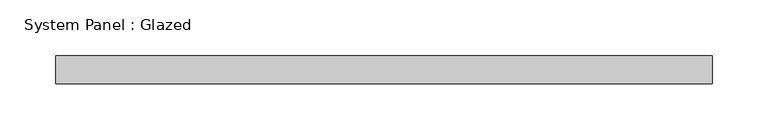
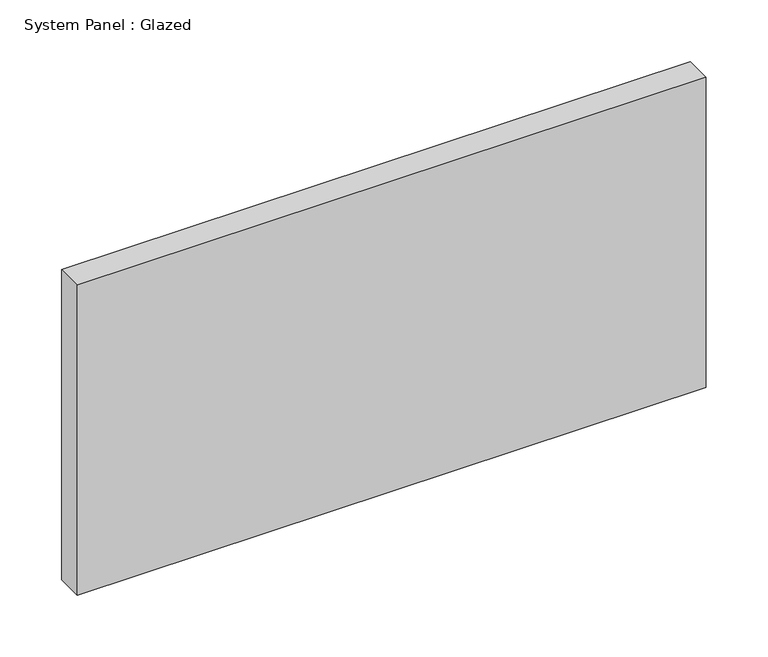
"""IFC4 building model written with IfcOpenShell, lengths in millimetres: plate geometry, System Panel : Glazed."""

from ifc_helpers import new_model, si_unit, origin, origin_with_axes, place, context, project, spatial, polyline, outline, extrude, source, transform, mapped, element, save


def system_panel_glazed_40061ca4(model_context):
    return source(origin(), model_context, "Body", "SweptSolid", [
        extrude(outline(polyline([(295.275, 19.05), (-295.275, 19.05), (-295.275, 44.45), (295.275, 44.45), (295.275, 19.05)])), origin_with_axes(), (0.0, 0.0, 1.0), 308.0546147),
    ])


if __name__ == "__main__":
    model = new_model("IFC4")
    model_context = context("Model", 3, world=origin())
    ifc_project = project(units=[si_unit("LENGTHUNIT", "METRE", prefix="MILLI")], contexts=[model_context])
    site = spatial("IfcSite", under=ifc_project)
    building = spatial("IfcBuilding", under=site)
    placement = place(None, origin())
    system_panel_glazed_shape = system_panel_glazed_40061ca4(model_context)
    element("IfcPlate", 1, ObjectType="System Panel : Glazed", at=placement, inside=building, context=model_context, shape_type="MappedRepresentation", body=[
        mapped(system_panel_glazed_shape, transform((0.0, 0.0, 0.0), x_axis=(1.0, 0.0, 0.0), y_axis=(0.0, 1.0, 0.0), z_axis=(0.0, 0.0, 1.0))),
    ])
    save(model, "model.ifc")

# Revit data of these elements
# Type "System Panel : Glazed"
#   Construction Type Id = "GSP4R"
#   Analytic Construction = "1/8 in Pilkington single glazing"
#   Visual Light Transmittance = 0.9
#   Solar Heat Gain Coefficient = 0.86
#   Heat Transfer Coefficient (U) = 1.18115 BTU/(h·ft²·°F)
#   Define Thermal Properties by = 1
# Element 1 (IfcPlate, "System Panel : Glazed")
#   Materials on its faces: "Glass"
# Materials
#   "Glass": class "Glass", colour RGB 0 128 192, transparency 0.75, Description = "Soda Lime Glass", Cost = 0
